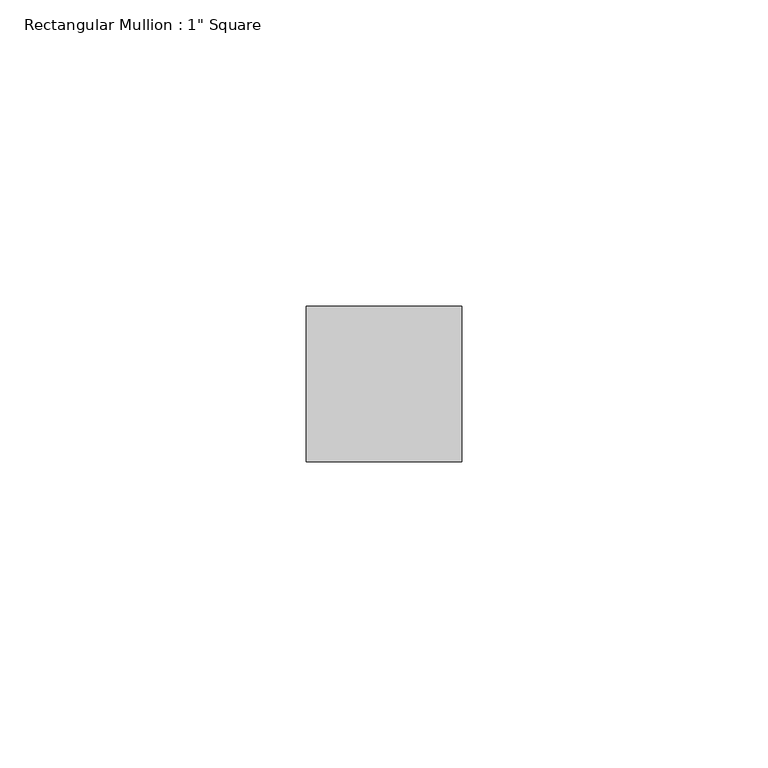
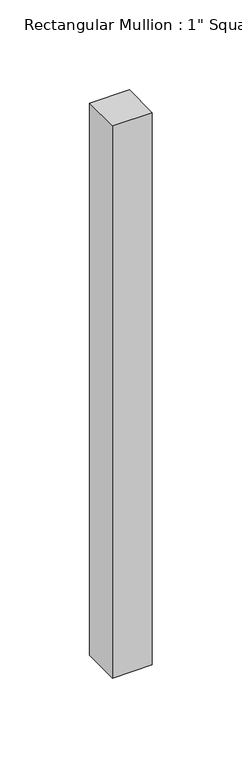
"""IFC4 building model written with IfcOpenShell, lengths in millimetres: member geometry."""

from ifc_helpers import new_model, si_unit, frame, origin, place, context, project, spatial, polyline, outline, extrude, source, transform, mapped, element, save


def member_34aa1075(model_context):
    return source(origin(), model_context, "Body", "SweptSolid", [
        extrude(outline(polyline([(0.0, 12.7), (0.0, -12.7), (-25.4, -12.7), (-25.4, 12.7), (0.0, 12.7)])), frame((0.0, 0.0, -374.65), z_axis=(0.0, 0.0, 1.0), x_axis=(1.0, 0.0, 0.0)), (0.0, 0.0, 1.0), 374.65),
    ])


if __name__ == "__main__":
    model = new_model("IFC4")
    model_context = context("Model", 3, world=origin())
    ifc_project = project(units=[si_unit("LENGTHUNIT", "METRE", prefix="MILLI")], contexts=[model_context])
    site = spatial("IfcSite", under=ifc_project)
    building = spatial("IfcBuilding", under=site)
    placement = place(None, origin())
    member_shape = member_34aa1075(model_context)
    element("IfcMember", 1, ObjectType="Rectangular Mullion : 1\" Square", at=placement, inside=building, context=model_context, shape_type="MappedRepresentation", body=[
        mapped(member_shape, transform((0.0, 0.0, 0.0), x_axis=(1.0, 0.0, 0.0), y_axis=(0.0, 1.0, 0.0), z_axis=(0.0, 0.0, 1.0))),
    ])
    save(model, "model.ifc")

# Revit data of these elements
# Type "Rectangular Mullion : 1\" Square"
#   built-in parameter 1007304 = 0.0833333 (stored number, unit not read)
#   built-in parameter 1007301 = 0.0416667 (stored number, unit not read)
#   built-in parameter 1007300 = 0.0416667 (stored number, unit not read)
